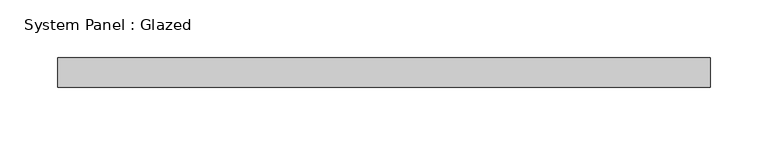
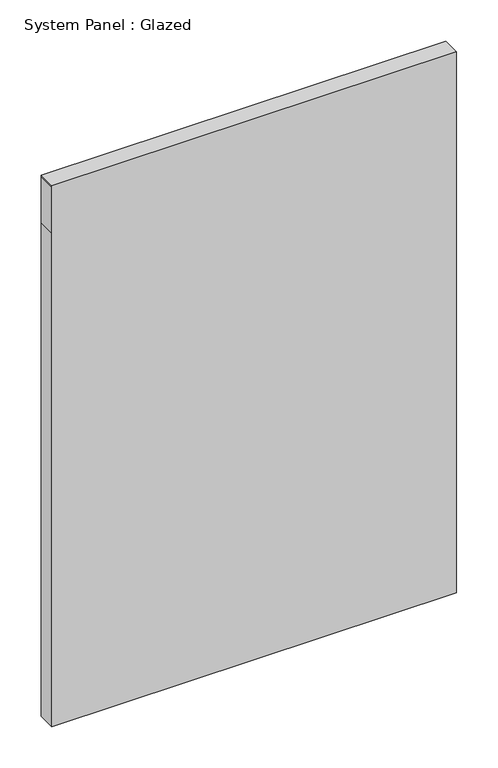
"""IFC4 building model written with IfcOpenShell, lengths in millimetres: plate geometry, System Panel : Glazed."""

from ifc_helpers import new_model, si_unit, frame, origin, place, context, project, spatial, polyline, outline, extrude, source, transform, mapped, element, save


def system_panel_glazed_871766ed(model_context):
    return source(origin(), model_context, "Body", "SweptSolid", [
        extrude(outline(polyline([(0.0, -282.575), (0.0, 282.575), (727.7941631, 282.575), (795.5274964, 282.575), (797.6441631, 282.575), (797.6441631, -282.575), (795.5274964, -282.575), (727.7941631, -282.575), (0.0, -282.575)])), frame((0.0, 19.05, 0.0), z_axis=(0.0, 1.0, 0.0), x_axis=(0.0, 0.0, 1.0)), (0.0, 0.0, 1.0), 25.4),
    ])


if __name__ == "__main__":
    model = new_model("IFC4")
    model_context = context("Model", 3, world=origin())
    ifc_project = project(units=[si_unit("LENGTHUNIT", "METRE", prefix="MILLI")], contexts=[model_context])
    site = spatial("IfcSite", under=ifc_project)
    building = spatial("IfcBuilding", under=site)
    placement = place(None, origin())
    system_panel_glazed_shape = system_panel_glazed_871766ed(model_context)
    element("IfcPlate", 1, ObjectType="System Panel : Glazed", at=placement, inside=building, context=model_context, shape_type="MappedRepresentation", body=[
        mapped(system_panel_glazed_shape, transform((0.0, 0.0, 0.0), x_axis=(1.0, 0.0, 0.0), y_axis=(0.0, 1.0, 0.0), z_axis=(0.0, 0.0, 1.0))),
    ])
    save(model, "model.ifc")

# Revit data of these elements
# Type "System Panel : Glazed"
#   Construction Type Id = "GSP4R"
#   Analytic Construction = "1/8 in Pilkington single glazing"
#   Visual Light Transmittance = 0.9
#   Solar Heat Gain Coefficient = 0.86
#   Heat Transfer Coefficient (U) = 1.18115 BTU/(h·ft²·°F)
#   Define Thermal Properties by = 1
# Element 1 (IfcPlate, "System Panel : Glazed")
#   Materials on its faces: "Glass"
# Materials
#   "Glass": class "Glass", colour RGB 0 128 192, transparency 0.75, Description = "Soda Lime Glass", Cost = 0
